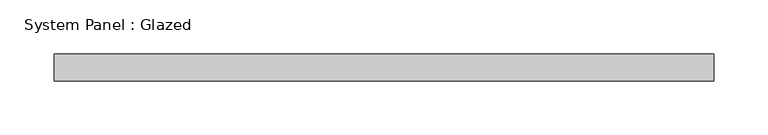
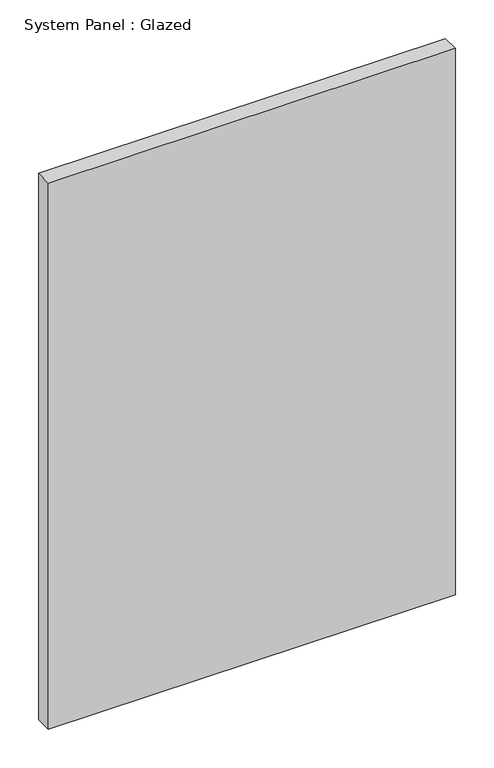
"""IFC4 building model written with IfcOpenShell, lengths in millimetres: plate geometry, System Panel : Glazed."""

from ifc_helpers import new_model, si_unit, origin, origin_with_axes, place, context, project, spatial, polyline, outline, extrude, source, transform, mapped, element, save


def system_panel_glazed_b26c39eb(model_context):
    return source(origin(), model_context, "Body", "SweptSolid", [
        extrude(outline(polyline([(304.8, 24.5), (-304.8, 24.5), (-304.8, 49.5), (304.8, 49.5), (304.8, 24.5)])), origin_with_axes(), (0.0, 0.0, 1.0), 864.4),
    ])


if __name__ == "__main__":
    model = new_model("IFC4")
    model_context = context("Model", 3, world=origin())
    ifc_project = project(units=[si_unit("LENGTHUNIT", "METRE", prefix="MILLI")], contexts=[model_context])
    site = spatial("IfcSite", under=ifc_project)
    building = spatial("IfcBuilding", under=site)
    placement = place(None, origin())
    system_panel_glazed_shape = system_panel_glazed_b26c39eb(model_context)
    element("IfcPlate", 1, ObjectType="System Panel : Glazed", at=placement, inside=building, context=model_context, shape_type="MappedRepresentation", body=[
        mapped(system_panel_glazed_shape, transform((0.0, 0.0, 0.0), x_axis=(1.0, 0.0, 0.0), y_axis=(0.0, 1.0, 0.0), z_axis=(0.0, 0.0, 1.0))),
    ])
    save(model, "model.ifc")

# Revit data of these elements
# Type "System Panel : Glazed"
#   Keynote = "H11"
#   Construction Type Id = "GSP4R"
#   Analytic Construction = "1/8 in Pilkington single glazing"
#   Visual Light Transmittance = 0.9
#   Solar Heat Gain Coefficient = 0.86
#   Heat Transfer Coefficient (U) = 6.7069 W/(m²·K)
#   Define Thermal Properties by = 1
# Element 1 (IfcPlate, "System Panel : Glazed")
#   Materials on its faces: "Glass"
# Materials
#   "Glass": class "Glass", colour RGB 0 128 192, transparency 0.9, Description = "Soda Lime Glass", Cost = 0
